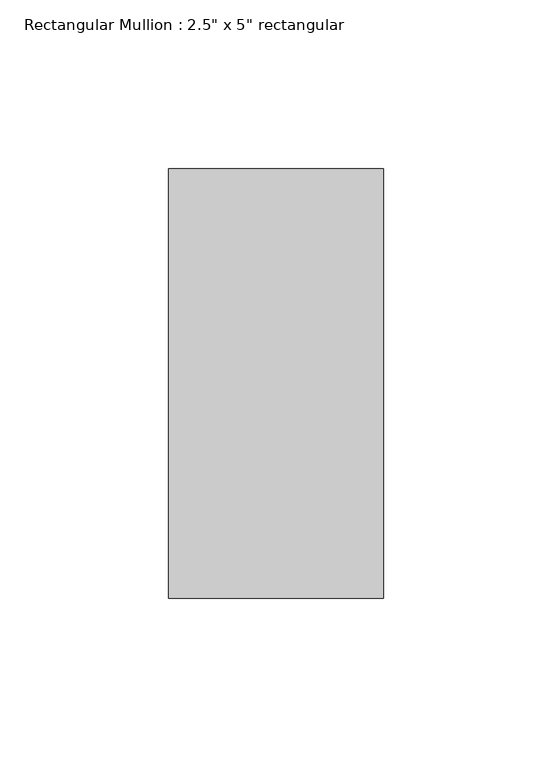
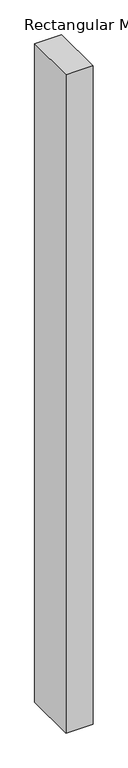
"""IFC4 building model written with IfcOpenShell, lengths in millimetres: member geometry."""

from ifc_helpers import new_model, si_unit, frame, origin, place, context, project, spatial, polyline, outline, extrude, source, transform, mapped, element, save


def member_fa50fb7e(model_context):
    return source(origin(), model_context, "Body", "SweptSolid", [
        extrude(outline(polyline([(31.75, 63.5), (31.75, -63.5), (-31.75, -63.5), (-31.75, 63.5), (31.75, 63.5)])), frame((0.0, 0.0, -1633.7500384), z_axis=(0.0, 0.0, 1.0), x_axis=(1.0, 0.0, 0.0)), (0.0, 0.0, 1.0), 1633.7500384),
    ])


if __name__ == "__main__":
    model = new_model("IFC4")
    model_context = context("Model", 3, world=origin())
    ifc_project = project(units=[si_unit("LENGTHUNIT", "METRE", prefix="MILLI")], contexts=[model_context])
    site = spatial("IfcSite", under=ifc_project)
    building = spatial("IfcBuilding", under=site)
    placement = place(None, origin())
    member_shape = member_fa50fb7e(model_context)
    element("IfcMember", 1, ObjectType="Rectangular Mullion : 2.5\" x 5\" rectangular", at=placement, inside=building, context=model_context, shape_type="MappedRepresentation", body=[
        mapped(member_shape, transform((0.0, 0.0, 0.0), x_axis=(1.0, 0.0, 0.0), y_axis=(0.0, 1.0, 0.0), z_axis=(0.0, 0.0, 1.0))),
    ])
    save(model, "model.ifc")

# Revit data of these elements
# Type "Rectangular Mullion : 2.5\" x 5\" rectangular"
#   built-in parameter 1007304 = 0.416667 (stored number, unit not read)
#   built-in parameter 1007301 = 0.104167 (stored number, unit not read)
#   built-in parameter 1007300 = 0.104167 (stored number, unit not read)
# Element 1 (IfcMember, "Rectangular Mullion : 2.5\" x 5\" rectangular")
#   Materials on its faces: "Aluminum"
# Materials
#   "Aluminum": class "Metal", colour RGB 247 247 247, transparency 0, Description = "Aluminum 6061", Cost = 0
